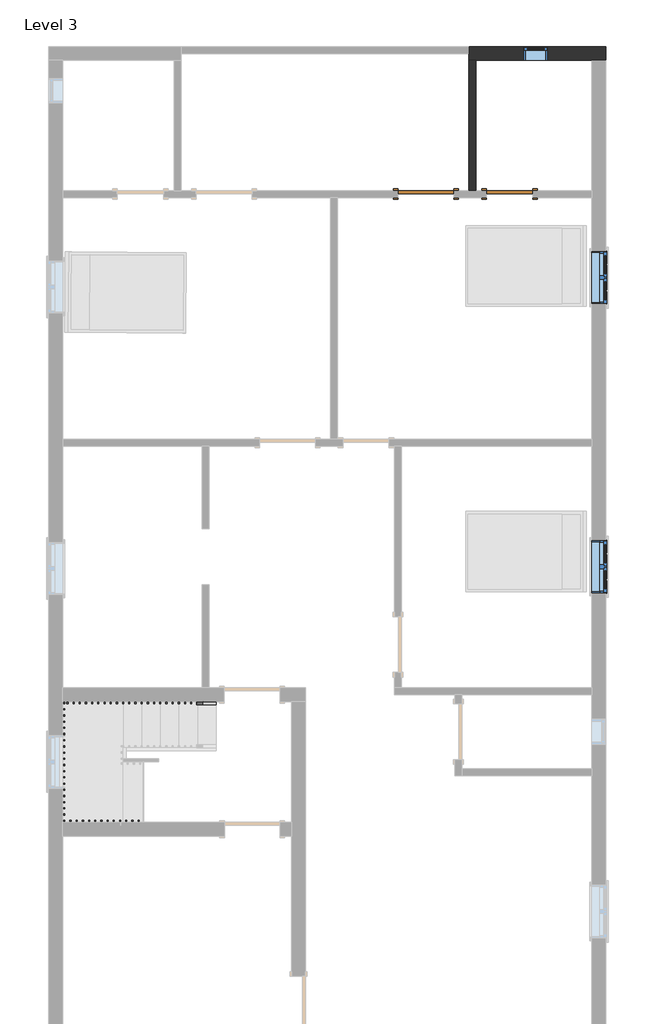
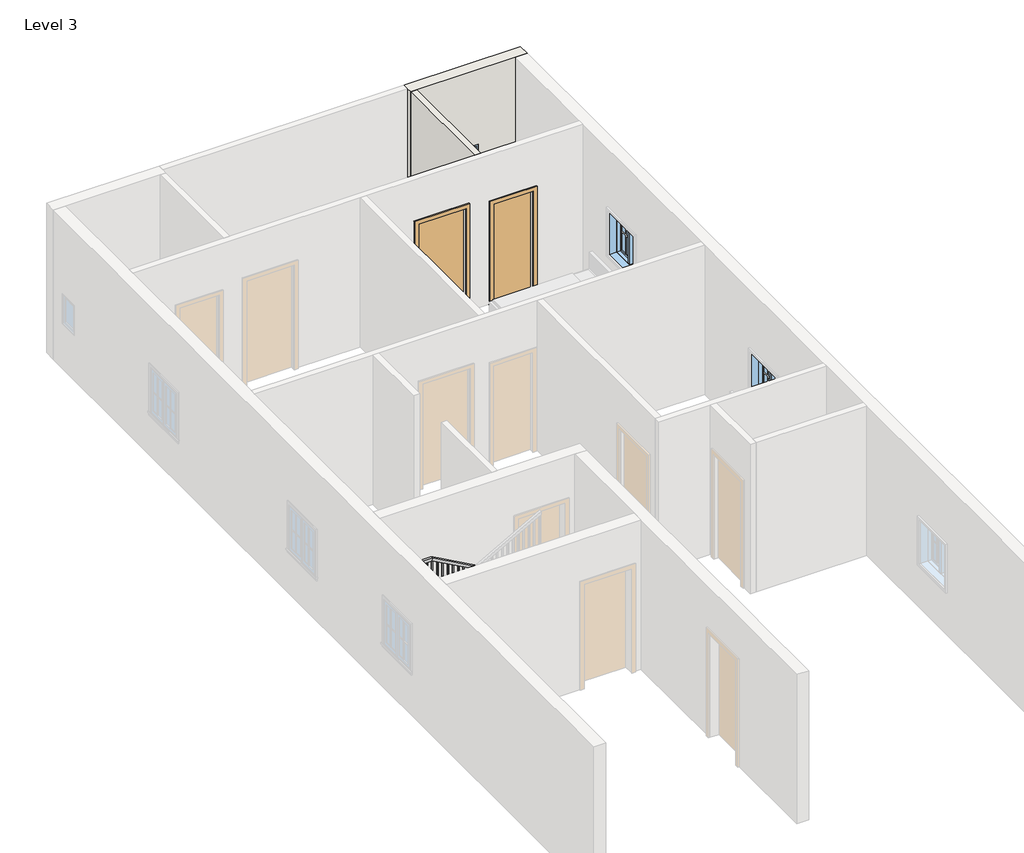
# One storey, part 2 of 3: 3 windows, 2 doors, 2 walls, 1 railing.
"""IFC4 building model written with IfcOpenShell, lengths in millimetres."""

from ifc_helpers import new_model, si_unit, frame, origin, place, context, project, spatial, polyline, outline, extrude, faceted_brep, transform, mapped, element, save
from components import door_f2b275c1, door_e5f9f3c4, window_aa618e30, window_339605e1

model = new_model("IFC4")

# Units and contexts
model_context = context("Model", 3, world=origin())
ifc_project = project(units=[si_unit("LENGTHUNIT", "METRE", prefix="MILLI")], contexts=[model_context])

# Site, building, storey
site = spatial("IfcSite", under=ifc_project)
building = spatial("IfcBuilding", under=site)
storey = spatial("IfcBuildingStorey", under=building, Name="Level 3", Elevation=3200.4)

# Doors
placement = place(None, origin())
door_shape = door_f2b275c1(model_context)
element("IfcDoor", 1, ObjectType="Single-Flush : 30\" x 80\"", at=placement, inside=storey, context=model_context, shape_type="MappedRepresentation", body=[
    mapped(door_shape, transform((1735.6084916, 8007.7072267, 3200.4), x_axis=(-1.0, 0.0, 0.0), y_axis=(0.0, -1.0, 0.0), z_axis=(0.0, 0.0, 1.0))),
])
door_2_shape = door_e5f9f3c4(model_context)
element("IfcDoor", 2, ObjectType="Single-Flush : 36\" x 84\"", at=placement, inside=storey, context=model_context, shape_type="MappedRepresentation", body=[
    mapped(door_2_shape, transform((364.0084916, 8007.7072267, 3200.4), x_axis=(1.0, 0.0, 0.0), y_axis=(0.0, 1.0, 0.0), z_axis=(0.0, 0.0, 1.0))),
])

# Railing
element("IfcRailing", 3, ObjectType="Handrail - Rectangular", at=placement, inside=storey, context=model_context, shape_type="SolidModel", body=[
    faceted_brep([(-3084.0415084, -367.9427733, 4284.1333333), (-3084.0415084, -367.9427733, 4226.020221), (-3084.0415084, -317.1427733, 4226.020221), (-3084.0415084, -317.1427733, 4284.1333333), (-4608.0415084, -367.9427733, 5130.8), (-4621.2051106, -367.9427733, 5080.0), (-4621.2051106, -317.1427733, 5080.0), (-4608.0415084, -317.1427733, 5130.8), (-5547.8415084, -367.9427733, 5130.8), (-5547.8415084, -367.9427733, 5080.0), (-5598.6415084, -317.1427733, 5080.0), (-5598.6415084, -317.1427733, 5130.8), (-5547.8415084, -2247.5427733, 5130.8), (-5547.8415084, -2247.5427733, 5080.0), (-5598.6415084, -2298.3427733, 5080.0), (-5598.6415084, -2298.3427733, 5130.8), (-4912.8415084, -2247.5427733, 5130.8), (-4899.6779062, -2247.5427733, 5080.0), (-4899.6779062, -2298.3427733, 5080.0), (-4912.8415084, -2298.3427733, 5130.8), (-3084.0415084, -2247.5427733, 6146.8), (-3084.0415084, -2298.3427733, 6146.8), (-3084.0415084, -2298.3427733, 6088.6868876), (-3084.0415084, -2247.5427733, 6088.6868876)], [[[0, 1, 2, 3]], [[1, 0, 4, 5]], [[2, 1, 5, 6]], [[3, 2, 6, 7]], [[0, 3, 7, 4]], [[5, 4, 8, 9]], [[6, 5, 9, 10]], [[7, 6, 10, 11]], [[4, 7, 11, 8]], [[9, 8, 12, 13]], [[10, 9, 13, 14]], [[11, 10, 14, 15]], [[8, 11, 15, 12]], [[13, 12, 16, 17]], [[14, 13, 17, 18]], [[15, 14, 18, 19]], [[12, 15, 19, 16]], [[20, 21, 22, 23]], [[17, 16, 20, 23]], [[18, 17, 23, 22]], [[19, 18, 22, 21]], [[16, 19, 21, 20]]]),
    extrude(outline(polyline([(6065.7563321, -3125.3165084), (6055.1729988, -3144.3665084), (5063.0666667, -3144.3665084), (5063.0666667, -3125.3165084), (6065.7563321, -3125.3165084)])), frame((0.0, -2282.4677733, 0.0), z_axis=(0.0, 1.0, 0.0), x_axis=(0.0, 0.0, 1.0)), (0.0, 0.0, 1.0), 19.05),
    extrude(outline(polyline([(6009.3118876, -3226.9165084), (5998.7285543, -3245.9665084), (5063.0666667, -3245.9665084), (5063.0666667, -3226.9165084), (6009.3118876, -3226.9165084)])), frame((0.0, -2282.4677733, 0.0), z_axis=(0.0, 1.0, 0.0), x_axis=(0.0, 0.0, 1.0)), (0.0, 0.0, 1.0), 19.05),
    extrude(outline(polyline([(5952.8674432, -3328.5165084), (5942.2841099, -3347.5665084), (5063.0666667, -3347.5665084), (5063.0666667, -3328.5165084), (5952.8674432, -3328.5165084)])), frame((0.0, -2282.4677733, 0.0), z_axis=(0.0, 1.0, 0.0), x_axis=(0.0, 0.0, 1.0)), (0.0, 0.0, 1.0), 19.05),
    extrude(outline(polyline([(5896.4229988, -3430.1165084), (5885.8396654, -3449.1665084), (4893.7333333, -3449.1665084), (4893.7333333, -3430.1165084), (5896.4229988, -3430.1165084)])), frame((0.0, -2282.4677733, 0.0), z_axis=(0.0, 1.0, 0.0), x_axis=(0.0, 0.0, 1.0)), (0.0, 0.0, 1.0), 19.05),
    extrude(outline(polyline([(5839.9785543, -3531.7165084), (5829.395221, -3550.7665084), (4893.7333333, -3550.7665084), (4893.7333333, -3531.7165084), (5839.9785543, -3531.7165084)])), frame((0.0, -2282.4677733, 0.0), z_axis=(0.0, 1.0, 0.0), x_axis=(0.0, 0.0, 1.0)), (0.0, 0.0, 1.0), 19.05),
    extrude(outline(polyline([(5783.5341099, -3633.3165084), (5772.9507765, -3652.3665084), (4893.7333333, -3652.3665084), (4893.7333333, -3633.3165084), (5783.5341099, -3633.3165084)])), frame((0.0, -2282.4677733, 0.0), z_axis=(0.0, 1.0, 0.0), x_axis=(0.0, 0.0, 1.0)), (0.0, 0.0, 1.0), 19.05),
    extrude(outline(polyline([(5727.0896654, -3734.9165084), (5716.5063321, -3753.9665084), (4724.4, -3753.9665084), (4724.4, -3734.9165084), (5727.0896654, -3734.9165084)])), frame((0.0, -2282.4677733, 0.0), z_axis=(0.0, 1.0, 0.0), x_axis=(0.0, 0.0, 1.0)), (0.0, 0.0, 1.0), 19.05),
    extrude(outline(polyline([(5670.645221, -3836.5165084), (5660.0618876, -3855.5665084), (4724.4, -3855.5665084), (4724.4, -3836.5165084), (5670.645221, -3836.5165084)])), frame((0.0, -2282.4677733, 0.0), z_axis=(0.0, 1.0, 0.0), x_axis=(0.0, 0.0, 1.0)), (0.0, 0.0, 1.0), 19.05),
    extrude(outline(polyline([(5614.2007765, -3938.1165084), (5603.6174432, -3957.1665084), (4724.4, -3957.1665084), (4724.4, -3938.1165084), (5614.2007765, -3938.1165084)])), frame((0.0, -2282.4677733, 0.0), z_axis=(0.0, 1.0, 0.0), x_axis=(0.0, 0.0, 1.0)), (0.0, 0.0, 1.0), 19.05),
    extrude(outline(polyline([(5557.7563321, -4039.7165084), (5547.1729988, -4058.7665084), (4555.0666667, -4058.7665084), (4555.0666667, -4039.7165084), (5557.7563321, -4039.7165084)])), frame((0.0, -2282.4677733, 0.0), z_axis=(0.0, 1.0, 0.0), x_axis=(0.0, 0.0, 1.0)), (0.0, 0.0, 1.0), 19.05),
    extrude(outline(polyline([(5501.3118876, -4141.3165084), (5490.7285543, -4160.3665084), (4555.0666667, -4160.3665084), (4555.0666667, -4141.3165084), (5501.3118876, -4141.3165084)])), frame((0.0, -2282.4677733, 0.0), z_axis=(0.0, 1.0, 0.0), x_axis=(0.0, 0.0, 1.0)), (0.0, 0.0, 1.0), 19.05),
    extrude(outline(polyline([(5444.8674432, -4242.9165084), (5434.2841099, -4261.9665084), (4555.0666667, -4261.9665084), (4555.0666667, -4242.9165084), (5444.8674432, -4242.9165084)])), frame((0.0, -2282.4677733, 0.0), z_axis=(0.0, 1.0, 0.0), x_axis=(0.0, 0.0, 1.0)), (0.0, 0.0, 1.0), 19.05),
    extrude(outline(polyline([(5388.4229988, -4344.5165084), (5377.8396654, -4363.5665084), (4385.7333333, -4363.5665084), (4385.7333333, -4344.5165084), (5388.4229988, -4344.5165084)])), frame((0.0, -2282.4677733, 0.0), z_axis=(0.0, 1.0, 0.0), x_axis=(0.0, 0.0, 1.0)), (0.0, 0.0, 1.0), 19.05),
    extrude(outline(polyline([(5331.9785543, -4446.1165084), (5321.395221, -4465.1665084), (4385.7333333, -4465.1665084), (4385.7333333, -4446.1165084), (5331.9785543, -4446.1165084)])), frame((0.0, -2282.4677733, 0.0), z_axis=(0.0, 1.0, 0.0), x_axis=(0.0, 0.0, 1.0)), (0.0, 0.0, 1.0), 19.05),
    extrude(outline(polyline([(5275.5341099, -4547.7165084), (5264.9507765, -4566.7665084), (4385.7333333, -4566.7665084), (4385.7333333, -4547.7165084), (5275.5341099, -4547.7165084)])), frame((0.0, -2282.4677733, 0.0), z_axis=(0.0, 1.0, 0.0), x_axis=(0.0, 0.0, 1.0)), (0.0, 0.0, 1.0), 19.05),
    extrude(outline(polyline([(5219.0896654, -4649.3165084), (5208.5063321, -4668.3665084), (4216.4, -4668.3665084), (4216.4, -4649.3165084), (5219.0896654, -4649.3165084)])), frame((0.0, -2282.4677733, 0.0), z_axis=(0.0, 1.0, 0.0), x_axis=(0.0, 0.0, 1.0)), (0.0, 0.0, 1.0), 19.05),
    extrude(outline(polyline([(5162.645221, -4750.9165084), (5152.0618876, -4769.9665084), (4216.4, -4769.9665084), (4216.4, -4750.9165084), (5162.645221, -4750.9165084)])), frame((0.0, -2282.4677733, 0.0), z_axis=(0.0, 1.0, 0.0), x_axis=(0.0, 0.0, 1.0)), (0.0, 0.0, 1.0), 19.05),
    extrude(outline(polyline([(5106.2007765, -4852.5165084), (5095.6174432, -4871.5665084), (4216.4, -4871.5665084), (4216.4, -4852.5165084), (5106.2007765, -4852.5165084)])), frame((0.0, -2282.4677733, 0.0), z_axis=(0.0, 1.0, 0.0), x_axis=(0.0, 0.0, 1.0)), (0.0, 0.0, 1.0), 19.05),
    extrude(outline(polyline([(-4973.1665084, -2282.4677733), (-4973.1665084, -2263.4177733), (-4954.1165084, -2263.4177733), (-4954.1165084, -2282.4677733), (-4973.1665084, -2282.4677733)])), frame((0.0, 0.0, 4216.4), z_axis=(0.0, 0.0, 1.0), x_axis=(1.0, 0.0, 0.0)), (0.0, 0.0, 1.0), 863.6),
    extrude(outline(polyline([(-5074.7665084, -2282.4677733), (-5074.7665084, -2263.4177733), (-5055.7165084, -2263.4177733), (-5055.7165084, -2282.4677733), (-5074.7665084, -2282.4677733)])), frame((0.0, 0.0, 4216.4), z_axis=(0.0, 0.0, 1.0), x_axis=(1.0, 0.0, 0.0)), (0.0, 0.0, 1.0), 863.6),
    extrude(outline(polyline([(-5176.3665084, -2282.4677733), (-5176.3665084, -2263.4177733), (-5157.3165084, -2263.4177733), (-5157.3165084, -2282.4677733), (-5176.3665084, -2282.4677733)])), frame((0.0, 0.0, 4216.4), z_axis=(0.0, 0.0, 1.0), x_axis=(1.0, 0.0, 0.0)), (0.0, 0.0, 1.0), 863.6),
    extrude(outline(polyline([(-5277.9665084, -2282.4677733), (-5277.9665084, -2263.4177733), (-5258.9165084, -2263.4177733), (-5258.9165084, -2282.4677733), (-5277.9665084, -2282.4677733)])), frame((0.0, 0.0, 4216.4), z_axis=(0.0, 0.0, 1.0), x_axis=(1.0, 0.0, 0.0)), (0.0, 0.0, 1.0), 863.6),
    extrude(outline(polyline([(-5379.5665084, -2282.4677733), (-5379.5665084, -2263.4177733), (-5360.5165084, -2263.4177733), (-5360.5165084, -2282.4677733), (-5379.5665084, -2282.4677733)])), frame((0.0, 0.0, 4216.4), z_axis=(0.0, 0.0, 1.0), x_axis=(1.0, 0.0, 0.0)), (0.0, 0.0, 1.0), 863.6),
    extrude(outline(polyline([(-5481.1665084, -2282.4677733), (-5481.1665084, -2263.4177733), (-5462.1165084, -2263.4177733), (-5462.1165084, -2282.4677733), (-5481.1665084, -2282.4677733)])), frame((0.0, 0.0, 4216.4), z_axis=(0.0, 0.0, 1.0), x_axis=(1.0, 0.0, 0.0)), (0.0, 0.0, 1.0), 863.6),
    extrude(outline(polyline([(-5582.7665084, -2161.8177733), (-5563.7165084, -2161.8177733), (-5563.7165084, -2180.8677733), (-5582.7665084, -2180.8677733), (-5582.7665084, -2161.8177733)])), frame((0.0, 0.0, 4216.4), z_axis=(0.0, 0.0, 1.0), x_axis=(1.0, 0.0, 0.0)), (0.0, 0.0, 1.0), 863.6),
    extrude(outline(polyline([(-5582.7665084, -2060.2177733), (-5563.7165084, -2060.2177733), (-5563.7165084, -2079.2677733), (-5582.7665084, -2079.2677733), (-5582.7665084, -2060.2177733)])), frame((0.0, 0.0, 4216.4), z_axis=(0.0, 0.0, 1.0), x_axis=(1.0, 0.0, 0.0)), (0.0, 0.0, 1.0), 863.6),
    extrude(outline(polyline([(-5582.7665084, -1958.6177733), (-5563.7165084, -1958.6177733), (-5563.7165084, -1977.6677733), (-5582.7665084, -1977.6677733), (-5582.7665084, -1958.6177733)])), frame((0.0, 0.0, 4216.4), z_axis=(0.0, 0.0, 1.0), x_axis=(1.0, 0.0, 0.0)), (0.0, 0.0, 1.0), 863.6),
    extrude(outline(polyline([(-5582.7665084, -1857.0177733), (-5563.7165084, -1857.0177733), (-5563.7165084, -1876.0677733), (-5582.7665084, -1876.0677733), (-5582.7665084, -1857.0177733)])), frame((0.0, 0.0, 4216.4), z_axis=(0.0, 0.0, 1.0), x_axis=(1.0, 0.0, 0.0)), (0.0, 0.0, 1.0), 863.6),
    extrude(outline(polyline([(-5582.7665084, -1755.4177733), (-5563.7165084, -1755.4177733), (-5563.7165084, -1774.4677733), (-5582.7665084, -1774.4677733), (-5582.7665084, -1755.4177733)])), frame((0.0, 0.0, 4216.4), z_axis=(0.0, 0.0, 1.0), x_axis=(1.0, 0.0, 0.0)), (0.0, 0.0, 1.0), 863.6),
    extrude(outline(polyline([(-5582.7665084, -1653.8177733), (-5563.7165084, -1653.8177733), (-5563.7165084, -1672.8677733), (-5582.7665084, -1672.8677733), (-5582.7665084, -1653.8177733)])), frame((0.0, 0.0, 4216.4), z_axis=(0.0, 0.0, 1.0), x_axis=(1.0, 0.0, 0.0)), (0.0, 0.0, 1.0), 863.6),
    extrude(outline(polyline([(-5582.7665084, -1552.2177733), (-5563.7165084, -1552.2177733), (-5563.7165084, -1571.2677733), (-5582.7665084, -1571.2677733), (-5582.7665084, -1552.2177733)])), frame((0.0, 0.0, 4216.4), z_axis=(0.0, 0.0, 1.0), x_axis=(1.0, 0.0, 0.0)), (0.0, 0.0, 1.0), 863.6),
    extrude(outline(polyline([(-5582.7665084, -1450.6177733), (-5563.7165084, -1450.6177733), (-5563.7165084, -1469.6677733), (-5582.7665084, -1469.6677733), (-5582.7665084, -1450.6177733)])), frame((0.0, 0.0, 4216.4), z_axis=(0.0, 0.0, 1.0), x_axis=(1.0, 0.0, 0.0)), (0.0, 0.0, 1.0), 863.6),
    extrude(outline(polyline([(-5582.7665084, -1349.0177733), (-5563.7165084, -1349.0177733), (-5563.7165084, -1368.0677733), (-5582.7665084, -1368.0677733), (-5582.7665084, -1349.0177733)])), frame((0.0, 0.0, 4216.4), z_axis=(0.0, 0.0, 1.0), x_axis=(1.0, 0.0, 0.0)), (0.0, 0.0, 1.0), 863.6),
    extrude(outline(polyline([(-5582.7665084, -1247.4177733), (-5563.7165084, -1247.4177733), (-5563.7165084, -1266.4677733), (-5582.7665084, -1266.4677733), (-5582.7665084, -1247.4177733)])), frame((0.0, 0.0, 4216.4), z_axis=(0.0, 0.0, 1.0), x_axis=(1.0, 0.0, 0.0)), (0.0, 0.0, 1.0), 863.6),
    extrude(outline(polyline([(-5582.7665084, -1145.8177733), (-5563.7165084, -1145.8177733), (-5563.7165084, -1164.8677733), (-5582.7665084, -1164.8677733), (-5582.7665084, -1145.8177733)])), frame((0.0, 0.0, 4216.4), z_axis=(0.0, 0.0, 1.0), x_axis=(1.0, 0.0, 0.0)), (0.0, 0.0, 1.0), 863.6),
    extrude(outline(polyline([(-5582.7665084, -1044.2177733), (-5563.7165084, -1044.2177733), (-5563.7165084, -1063.2677733), (-5582.7665084, -1063.2677733), (-5582.7665084, -1044.2177733)])), frame((0.0, 0.0, 4216.4), z_axis=(0.0, 0.0, 1.0), x_axis=(1.0, 0.0, 0.0)), (0.0, 0.0, 1.0), 863.6),
    extrude(outline(polyline([(-5582.7665084, -942.6177733), (-5563.7165084, -942.6177733), (-5563.7165084, -961.6677733), (-5582.7665084, -961.6677733), (-5582.7665084, -942.6177733)])), frame((0.0, 0.0, 4216.4), z_axis=(0.0, 0.0, 1.0), x_axis=(1.0, 0.0, 0.0)), (0.0, 0.0, 1.0), 863.6),
    extrude(outline(polyline([(-5582.7665084, -841.0177733), (-5563.7165084, -841.0177733), (-5563.7165084, -860.0677733), (-5582.7665084, -860.0677733), (-5582.7665084, -841.0177733)])), frame((0.0, 0.0, 4216.4), z_axis=(0.0, 0.0, 1.0), x_axis=(1.0, 0.0, 0.0)), (0.0, 0.0, 1.0), 863.6),
    extrude(outline(polyline([(-5582.7665084, -739.4177733), (-5563.7165084, -739.4177733), (-5563.7165084, -758.4677733), (-5582.7665084, -758.4677733), (-5582.7665084, -739.4177733)])), frame((0.0, 0.0, 4216.4), z_axis=(0.0, 0.0, 1.0), x_axis=(1.0, 0.0, 0.0)), (0.0, 0.0, 1.0), 863.6),
    extrude(outline(polyline([(-5582.7665084, -637.8177733), (-5563.7165084, -637.8177733), (-5563.7165084, -656.8677733), (-5582.7665084, -656.8677733), (-5582.7665084, -637.8177733)])), frame((0.0, 0.0, 4216.4), z_axis=(0.0, 0.0, 1.0), x_axis=(1.0, 0.0, 0.0)), (0.0, 0.0, 1.0), 863.6),
    extrude(outline(polyline([(-5582.7665084, -536.2177733), (-5563.7165084, -536.2177733), (-5563.7165084, -555.2677733), (-5582.7665084, -555.2677733), (-5582.7665084, -536.2177733)])), frame((0.0, 0.0, 4216.4), z_axis=(0.0, 0.0, 1.0), x_axis=(1.0, 0.0, 0.0)), (0.0, 0.0, 1.0), 863.6),
    extrude(outline(polyline([(-5582.7665084, -434.6177733), (-5563.7165084, -434.6177733), (-5563.7165084, -453.6677733), (-5582.7665084, -453.6677733), (-5582.7665084, -434.6177733)])), frame((0.0, 0.0, 4216.4), z_axis=(0.0, 0.0, 1.0), x_axis=(1.0, 0.0, 0.0)), (0.0, 0.0, 1.0), 863.6),
    extrude(outline(polyline([(-5512.9165084, -333.0177733), (-5512.9165084, -352.0677733), (-5531.9665084, -352.0677733), (-5531.9665084, -333.0177733), (-5512.9165084, -333.0177733)])), frame((0.0, 0.0, 4216.4), z_axis=(0.0, 0.0, 1.0), x_axis=(1.0, 0.0, 0.0)), (0.0, 0.0, 1.0), 863.6),
    extrude(outline(polyline([(-5411.3165084, -333.0177733), (-5411.3165084, -352.0677733), (-5430.3665084, -352.0677733), (-5430.3665084, -333.0177733), (-5411.3165084, -333.0177733)])), frame((0.0, 0.0, 4216.4), z_axis=(0.0, 0.0, 1.0), x_axis=(1.0, 0.0, 0.0)), (0.0, 0.0, 1.0), 863.6),
    extrude(outline(polyline([(-5309.7165084, -333.0177733), (-5309.7165084, -352.0677733), (-5328.7665084, -352.0677733), (-5328.7665084, -333.0177733), (-5309.7165084, -333.0177733)])), frame((0.0, 0.0, 4216.4), z_axis=(0.0, 0.0, 1.0), x_axis=(1.0, 0.0, 0.0)), (0.0, 0.0, 1.0), 863.6),
    extrude(outline(polyline([(-5208.1165084, -333.0177733), (-5208.1165084, -352.0677733), (-5227.1665084, -352.0677733), (-5227.1665084, -333.0177733), (-5208.1165084, -333.0177733)])), frame((0.0, 0.0, 4216.4), z_axis=(0.0, 0.0, 1.0), x_axis=(1.0, 0.0, 0.0)), (0.0, 0.0, 1.0), 863.6),
    extrude(outline(polyline([(-5106.5165084, -333.0177733), (-5106.5165084, -352.0677733), (-5125.5665084, -352.0677733), (-5125.5665084, -333.0177733), (-5106.5165084, -333.0177733)])), frame((0.0, 0.0, 4216.4), z_axis=(0.0, 0.0, 1.0), x_axis=(1.0, 0.0, 0.0)), (0.0, 0.0, 1.0), 863.6),
    extrude(outline(polyline([(-5004.9165084, -333.0177733), (-5004.9165084, -352.0677733), (-5023.9665084, -352.0677733), (-5023.9665084, -333.0177733), (-5004.9165084, -333.0177733)])), frame((0.0, 0.0, 4216.4), z_axis=(0.0, 0.0, 1.0), x_axis=(1.0, 0.0, 0.0)), (0.0, 0.0, 1.0), 863.6),
    extrude(outline(polyline([(-4903.3165084, -333.0177733), (-4903.3165084, -352.0677733), (-4922.3665084, -352.0677733), (-4922.3665084, -333.0177733), (-4903.3165084, -333.0177733)])), frame((0.0, 0.0, 4216.4), z_axis=(0.0, 0.0, 1.0), x_axis=(1.0, 0.0, 0.0)), (0.0, 0.0, 1.0), 863.6),
    extrude(outline(polyline([(-4801.7165084, -333.0177733), (-4801.7165084, -352.0677733), (-4820.7665084, -352.0677733), (-4820.7665084, -333.0177733), (-4801.7165084, -333.0177733)])), frame((0.0, 0.0, 4216.4), z_axis=(0.0, 0.0, 1.0), x_axis=(1.0, 0.0, 0.0)), (0.0, 0.0, 1.0), 863.6),
    extrude(outline(polyline([(-4700.1165084, -333.0177733), (-4700.1165084, -352.0677733), (-4719.1665084, -352.0677733), (-4719.1665084, -333.0177733), (-4700.1165084, -333.0177733)])), frame((0.0, 0.0, 4216.4), z_axis=(0.0, 0.0, 1.0), x_axis=(1.0, 0.0, 0.0)), (0.0, 0.0, 1.0), 863.6),
    extrude(outline(polyline([(5067.395221, -4598.5165084), (5077.9785543, -4617.5665084), (4216.4, -4617.5665084), (4216.4, -4598.5165084), (5067.395221, -4598.5165084)])), frame((0.0, -352.0677733, 0.0), z_axis=(0.0, 1.0, 0.0), x_axis=(0.0, 0.0, 1.0)), (0.0, 0.0, 1.0), 19.05),
    extrude(outline(polyline([(5010.9507765, -4496.9165084), (5021.5341099, -4515.9665084), (4047.0666667, -4515.9665084), (4047.0666667, -4496.9165084), (5010.9507765, -4496.9165084)])), frame((0.0, -352.0677733, 0.0), z_axis=(0.0, 1.0, 0.0), x_axis=(0.0, 0.0, 1.0)), (0.0, 0.0, 1.0), 19.05),
    extrude(outline(polyline([(4954.5063321, -4395.3165084), (4965.0896654, -4414.3665084), (4047.0666667, -4414.3665084), (4047.0666667, -4395.3165084), (4954.5063321, -4395.3165084)])), frame((0.0, -352.0677733, 0.0), z_axis=(0.0, 1.0, 0.0), x_axis=(0.0, 0.0, 1.0)), (0.0, 0.0, 1.0), 19.05),
    extrude(outline(polyline([(4898.0618876, -4293.7165084), (4908.645221, -4312.7665084), (4047.0666667, -4312.7665084), (4047.0666667, -4293.7165084), (4898.0618876, -4293.7165084)])), frame((0.0, -352.0677733, 0.0), z_axis=(0.0, 1.0, 0.0), x_axis=(0.0, 0.0, 1.0)), (0.0, 0.0, 1.0), 19.05),
    extrude(outline(polyline([(4841.6174432, -4192.1165084), (4852.2007765, -4211.1665084), (3877.7333333, -4211.1665084), (3877.7333333, -4192.1165084), (4841.6174432, -4192.1165084)])), frame((0.0, -352.0677733, 0.0), z_axis=(0.0, 1.0, 0.0), x_axis=(0.0, 0.0, 1.0)), (0.0, 0.0, 1.0), 19.05),
    extrude(outline(polyline([(4785.1729988, -4090.5165084), (4795.7563321, -4109.5665084), (3877.7333333, -4109.5665084), (3877.7333333, -4090.5165084), (4785.1729988, -4090.5165084)])), frame((0.0, -352.0677733, 0.0), z_axis=(0.0, 1.0, 0.0), x_axis=(0.0, 0.0, 1.0)), (0.0, 0.0, 1.0), 19.05),
    extrude(outline(polyline([(4728.7285543, -3988.9165084), (4739.3118876, -4007.9665084), (3877.7333333, -4007.9665084), (3877.7333333, -3988.9165084), (4728.7285543, -3988.9165084)])), frame((0.0, -352.0677733, 0.0), z_axis=(0.0, 1.0, 0.0), x_axis=(0.0, 0.0, 1.0)), (0.0, 0.0, 1.0), 19.05),
    extrude(outline(polyline([(4672.2841099, -3887.3165084), (4682.8674432, -3906.3665084), (3708.4, -3906.3665084), (3708.4, -3887.3165084), (4672.2841099, -3887.3165084)])), frame((0.0, -352.0677733, 0.0), z_axis=(0.0, 1.0, 0.0), x_axis=(0.0, 0.0, 1.0)), (0.0, 0.0, 1.0), 19.05),
    extrude(outline(polyline([(4615.8396654, -3785.7165084), (4626.4229988, -3804.7665084), (3708.4, -3804.7665084), (3708.4, -3785.7165084), (4615.8396654, -3785.7165084)])), frame((0.0, -352.0677733, 0.0), z_axis=(0.0, 1.0, 0.0), x_axis=(0.0, 0.0, 1.0)), (0.0, 0.0, 1.0), 19.05),
    extrude(outline(polyline([(4559.395221, -3684.1165084), (4569.9785543, -3703.1665084), (3708.4, -3703.1665084), (3708.4, -3684.1165084), (4559.395221, -3684.1165084)])), frame((0.0, -352.0677733, 0.0), z_axis=(0.0, 1.0, 0.0), x_axis=(0.0, 0.0, 1.0)), (0.0, 0.0, 1.0), 19.05),
    extrude(outline(polyline([(4502.9507765, -3582.5165084), (4513.5341099, -3601.5665084), (3539.0666667, -3601.5665084), (3539.0666667, -3582.5165084), (4502.9507765, -3582.5165084)])), frame((0.0, -352.0677733, 0.0), z_axis=(0.0, 1.0, 0.0), x_axis=(0.0, 0.0, 1.0)), (0.0, 0.0, 1.0), 19.05),
    extrude(outline(polyline([(4446.5063321, -3480.9165084), (4457.0896654, -3499.9665084), (3539.0666667, -3499.9665084), (3539.0666667, -3480.9165084), (4446.5063321, -3480.9165084)])), frame((0.0, -352.0677733, 0.0), z_axis=(0.0, 1.0, 0.0), x_axis=(0.0, 0.0, 1.0)), (0.0, 0.0, 1.0), 19.05),
    extrude(outline(polyline([(4390.0618876, -3379.3165084), (4400.645221, -3398.3665084), (3539.0666667, -3398.3665084), (3539.0666667, -3379.3165084), (4390.0618876, -3379.3165084)])), frame((0.0, -352.0677733, 0.0), z_axis=(0.0, 1.0, 0.0), x_axis=(0.0, 0.0, 1.0)), (0.0, 0.0, 1.0), 19.05),
    extrude(outline(polyline([(4333.6174432, -3277.7165084), (4344.2007765, -3296.7665084), (3369.7333333, -3296.7665084), (3369.7333333, -3277.7165084), (4333.6174432, -3277.7165084)])), frame((0.0, -352.0677733, 0.0), z_axis=(0.0, 1.0, 0.0), x_axis=(0.0, 0.0, 1.0)), (0.0, 0.0, 1.0), 19.05),
    extrude(outline(polyline([(4277.1729988, -3176.1165084), (4287.7563321, -3195.1665084), (3369.7333333, -3195.1665084), (3369.7333333, -3176.1165084), (4277.1729988, -3176.1165084)])), frame((0.0, -352.0677733, 0.0), z_axis=(0.0, 1.0, 0.0), x_axis=(0.0, 0.0, 1.0)), (0.0, 0.0, 1.0), 19.05),
    extrude(outline(polyline([(-5582.7665084, -2263.4177733), (-5563.7165084, -2263.4177733), (-5563.7165084, -2282.4677733), (-5582.7665084, -2282.4677733), (-5582.7665084, -2263.4177733)])), frame((0.0, 0.0, 4216.4), z_axis=(0.0, 0.0, 1.0), x_axis=(1.0, 0.0, 0.0)), (0.0, 0.0, 1.0), 863.6),
    extrude(outline(polyline([(-5563.7165084, -333.0177733), (-5563.7165084, -352.0677733), (-5582.7665084, -352.0677733), (-5582.7665084, -333.0177733), (-5563.7165084, -333.0177733)])), frame((0.0, 0.0, 4216.4), z_axis=(0.0, 0.0, 1.0), x_axis=(1.0, 0.0, 0.0)), (0.0, 0.0, 1.0), 863.6),
    extrude(outline(polyline([(6088.6868876, -3084.0415084), (6078.1035543, -3103.0915084), (5063.0666667, -3103.0915084), (5063.0666667, -3084.0415084), (6088.6868876, -3084.0415084)])), frame((0.0, -2282.4677733, 0.0), z_axis=(0.0, 1.0, 0.0), x_axis=(0.0, 0.0, 1.0)), (0.0, 0.0, 1.0), 19.05),
    extrude(outline(polyline([(4226.020221, -3084.0415084), (4236.6035543, -3103.0915084), (3369.7333333, -3103.0915084), (3369.7333333, -3084.0415084), (4226.020221, -3084.0415084)])), frame((0.0, -352.0677733, 0.0), z_axis=(0.0, 1.0, 0.0), x_axis=(0.0, 0.0, 1.0)), (0.0, 0.0, 1.0), 19.05),
])

# Walls
element("IfcWall", 4, ObjectType="WALL4.5\"", at=placement, inside=storey, context=model_context, shape_type="SweptSolid", body=[
    extrude(outline(polyline([(1068.8584916, 8064.8572267), (1068.8584916, 10198.4572267), (1183.1584916, 10198.4572267), (1183.1584916, 8064.8572267), (1068.8584916, 8064.8572267)])), frame((0.0, 0.0, 3200.4), z_axis=(0.0, 0.0, 1.0), x_axis=(1.0, 0.0, 0.0)), (0.0, 0.0, 1.0), 3048.0),
])
element("IfcWall", 5, ObjectType="WALL9\"", at=placement, inside=storey, context=model_context, shape_type="Brep", body=[
    faceted_brep([(1068.8584916, 10198.4572267, 3200.4), (1183.1584916, 10198.4572267, 3200.4), (3088.1584916, 10198.4572267, 3200.4), (3316.7584916, 10198.4572267, 3200.4), (3316.7584916, 10198.4572267, 6248.4), (3088.1584916, 10198.4572267, 6248.4), (1183.1584916, 10198.4572267, 6248.4), (1068.8584916, 10198.4572267, 6248.4), (2367.4334916, 10198.4572267, 4724.4), (2367.4334916, 10198.4572267, 4114.8), (1961.0334916, 10198.4572267, 4114.8), (1961.0334916, 10198.4572267, 4724.4), (1068.8584916, 10427.0572267, 3200.4), (1068.8584916, 10427.0572267, 6248.4), (3316.7584916, 10427.0572267, 6248.4), (3316.7584916, 10427.0572267, 3200.4), (2367.4334916, 10427.0572267, 4724.4), (1961.0334916, 10427.0572267, 4724.4), (1961.0334916, 10427.0572267, 4114.8), (2367.4334916, 10427.0572267, 4114.8), (1068.8584916, 10312.7572267, 3200.4), (1068.8584916, 10312.7572267, 6248.4)], [[[0, 1, 2, 3, 4, 5, 6, 7], [8, 9, 10, 11]], [[12, 13, 14, 15], [16, 17, 18, 19]], [[3, 2, 1, 0, 20, 12, 15]], [[4, 3, 15, 14]], [[0, 7, 21, 13, 12, 20]], [[9, 8, 16, 19]], [[10, 9, 19, 18]], [[11, 10, 18, 17]], [[8, 11, 17, 16]], [[7, 6, 5, 4, 14, 13, 21]]]),
])

# Windows
window_shape = window_aa618e30(model_context)
element("IfcWindow", 6, ObjectType="Fixed : 16\" x 24\"", at=placement, inside=storey, context=model_context, shape_type="MappedRepresentation", body=[
    mapped(window_shape, transform((2202.3334916, 10312.7572267, 3200.4), x_axis=(1.0, 0.0, 0.0), y_axis=(0.0, 1.0, 0.0), z_axis=(0.0, 0.0, 1.0))),
])
window_2_shape = window_339605e1(model_context)
element("IfcWindow", 7, ObjectType="Window-Casement-Double : 34\" x 36\"", at=placement, inside=storey, context=model_context, shape_type="MappedRepresentation", body=[
    mapped(window_2_shape, transform((3202.4584916, 6636.1072267, 3200.4), x_axis=(0.0, -1.0, 0.0), y_axis=(1.0, 0.0, 0.0), z_axis=(0.0, 0.0, 1.0))),
])
element("IfcWindow", 8, ObjectType="Window-Casement-Double : 34\" x 36\"", at=placement, inside=storey, context=model_context, shape_type="MappedRepresentation", body=[
    mapped(window_2_shape, transform((3202.4584916, 1892.6572267, 3200.4), x_axis=(0.0, -1.0, 0.0), y_axis=(1.0, 0.0, 0.0), z_axis=(0.0, 0.0, 1.0))),
])

save(model, "model.ifc")

# Revit data of these elements
# Type "Single-Flush : 30\" x 80\""
#   Type Mark = "5"
#   Construction Type Id = "MDOOR"
#   Assembly Code = "C1020"
#   Analytic Construction = "Metal"
#   Thickness = 0' - 2"
#   Heat Transfer Coefficient (U) = 0.651978 BTU/(h·ft²·°F)
#   Height = 6' - 8"
#   Trim Projection Ext = 0' - 1"
#   Trim Projection Int = 0' - 1"
#   Trim Width = 0' - 3"
#   Width = 2' - 6"
#   Define Thermal Properties by = 1
#   Define Thermal Properties by = 1
#   Door Material = Door - Panel
#   Frame Material = Door - Frame
#   Visual Light Transmittance = 0
#   Solar Heat Gain Coefficient = 0
#   Function = (empty or 0)
#   Wall Closure = (empty or 0)
# Type "Single-Flush : 36\" x 84\""
#   Type Mark = "1"
#   Construction Type Id = "MDOOR"
#   Assembly Code = "C1020"
#   Analytic Construction = "Metal"
#   Thickness = 0' - 2"
#   Heat Transfer Coefficient (U) = 0.651978 BTU/(h·ft²·°F)
#   Height = 7' - 0"
#   Trim Projection Ext = 0' - 1"
#   Trim Projection Int = 0' - 1"
#   Trim Width = 0' - 3"
#   Width = 3' - 0"
#   Define Thermal Properties by = 1
#   Define Thermal Properties by = 1
#   Door Material = Door - Panel
#   Frame Material = Door - Frame
#   Visual Light Transmittance = 0
#   Solar Heat Gain Coefficient = 0
#   Function = (empty or 0)
#   Wall Closure = (empty or 0)
# Type "Handrail - Rectangular"
#   Assembly Code = "C2010400"
#   built-in parameter 1008612 = 0.0416667 (stored number, unit not read)
#   built-in parameter 1008611 = 0.0416667 (stored number, unit not read)
#   built-in parameter 1008609 = 0.333333 (stored number, unit not read)
#   built-in parameter 1008604 = 0.166667 (stored number, unit not read)
#   built-in parameter 1008603 = 0.166667 (stored number, unit not read)
#   Railing Height = 3' - 0"
#   built-in parameter 1008630 = 2
#   built-in parameter 1008610 = 2
#   built-in parameter 1008618 = Baluster - Square : 3/4"
# Type "WALL4.5\""
#   Assembly Code = "B2010"
#   Layers, outside or top first: 0' - 4 1/2" no material (function 1)
# Type "WALL9\""
#   Assembly Code = "B2010"
#   Layers, outside or top first: 0' - 9" no material (function 1)
# Type "Fixed : 16\" x 24\""
#   Type Mark = "4"
#   Construction Type Id = "GSP4R"
#   Assembly Code = "B2020100"
#   Analytic Construction = "1/8 in Pilkington single glazing"
#   Visual Light Transmittance = 0.9
#   Solar Heat Gain Coefficient = 0.78
#   Heat Transfer Coefficient (U) = 0.6496 BTU/(h·ft²·°F)
#   Height = 2' - 0"
#   Default Sill Height = 3' - 0"
#   Width = 1' - 4"
#   Window Inset = 0' - 0 3/4"
#   Define Thermal Properties by = 1
#   Define Thermal Properties by = 1
#   Glass Pane Material = Glass
#   Sash Material = Sash
#   Wall Closure = (empty or 0)
# Type "Window-Casement-Double : 34\" x 36\""
#   Type Mark = "14"
#   Fire Rating = "0.5h"
#   Assembly Code = "B2020100"
#   Analytic Construction = "Double glazing - domestic"
#   Frame Extension [instance default] = 0' - 0 1/4"
#   Window Inset [instance default] = 0' - 0"
#   Wall Thickness [instance default] = 0' - 6"
#   Interior Wall Closure [instance default] = 0' - 2 1/4"
#   Half Width = 1' - 5"
#   Visual Light Transmittance = 0.81
#   Thermal Resistance (R) = 1.8146 (h·ft²·°F)/BTU
#   Solar Heat Gain Coefficient = 0.76
#   Rough Width = 2' - 10 1/2"
#   Rough Height = 3' - 0 1/2"
#   Height = 3' - 0"
#   Heat Transfer Coefficient (U) = 0.5511 BTU/(h·ft²·°F)
#   Exterior Wall Closure [instance default] = 0' - 1 1/4"
#   Extension Jamb [instance default] = 0' - 2 1/4"
#   Default Sill Height = 3' - 0"
#   Width = 2' - 10"
#   Define Thermal Properties by = 0
#   Muntin Visibility = yes
#   Interior Trim Visibility [instance default] = yes
#   Exterior Trim Visibility [instance default] = yes
#   Extension Jamb Visibility [instance default] = yes
#   Interior Trim Material = Wood - Stained
#   Muntin Pattern = Muntin Pattern_2x2 : Muntin Pattern_2x2
#   Interior Trim = Trim-Window-Interior-Flat : Picture Frame
#   Interior Frame Material = Wood - Stained
#   Glass Panel Material = Glass
#   Exterior Trim Material = Clad - White
#   Exterior Trim = Trim-Window-Exterior-Flat : with Sill
#   Exterior Frame Material = Clad - White
#   Wall Closure = (empty or 0)
# Element 1 (IfcDoor, "Single-Flush : 30\" x 80\"")
#   Phase Created = New Construction
#   Materials on its faces: "Door - Frame", "Door - Panel"
# Element 2 (IfcDoor, "Single-Flush : 36\" x 84\"")
#   Phase Created = New Construction
#   Materials on its faces: "Door - Frame", "Door - Panel"
# Element 3 (IfcRailing, "Handrail - Rectangular")
#   Phase Created = New Construction
# Element 4 (IfcWall, "WALL4.5\"")
#   Top Offset = 0' - 0"
#   Base Offset = 0' - 0"
#   Unconnected Height = 10' - 0"
#   wall height = 10' - 0"
#   Phase Created = New Construction
#   Base Constraint = Level 3
#   Materials on its faces: "Default Wall", "Wood Planks"
# Element 5 (IfcWall, "WALL9\"")
#   Top Offset = 0' - 0"
#   Base Offset = 0' - 0"
#   Unconnected Height = 10' - 0"
#   wall height = 10' - 0"
#   Phase Created = New Construction
#   Base Constraint = Level 3
#   Materials on its faces: "Default Wall", "Wood Planks"
# Element 6 (IfcWindow, "Fixed : 16\" x 24\"")
#   Mark = "11"
#   Phase Created = New Construction
#   Materials on its faces: "Sash", "Glass"
# Element 7 (IfcWindow, "Window-Casement-Double : 34\" x 36\"")
#   Mark = "13"
#   Window Inset = 0' - 0"
#   Interior Wall Closure = 0' - 2 1/4"
#   Frame Extension = 0' - 0 1/4"
#   Exterior Wall Closure = 0' - 1 1/4"
#   Interior Trim Visibility = yes
#   Exterior Trim Visibility = yes
#   Phase Created = New Construction
#   Materials on its faces: "Wood - Stained", "Glass", "Clad - White"
# Element 8 (IfcWindow, "Window-Casement-Double : 34\" x 36\"")
#   Mark = "14"
#   Window Inset = 0' - 0"
#   Interior Wall Closure = 0' - 2 1/4"
#   Frame Extension = 0' - 0 1/4"
#   Exterior Wall Closure = 0' - 1 1/4"
#   Interior Trim Visibility = yes
#   Exterior Trim Visibility = yes
#   Phase Created = New Construction
#   Materials on its faces: "Wood - Stained", "Glass", "Clad - White"
# Materials
#   "Door - Panel": class "Wood", colour RGB 210 159 95, transparency 0, Cost = 0
#   "Door - Frame": colour RGB 118 70 51, transparency 0, Cost = 0
#   "Glass": class "Glass", colour RGB 0 128 192, transparency 0.75, Description = "Soda Lime Glass", Cost = 0
#   "Sash": class "Wood", colour RGB 224 178 126, transparency 0, Cost = 0
#   "Wood - Stained": class "Wood", colour RGB 224 178 126, transparency 0, Cost = 0
#   "Clad - White": class "Wood", colour RGB 242 242 238, transparency 0, Cost = 0
#   "Default Wall": colour RGB 128 128 128, transparency 0, Cost = 0
#   "Wood Planks": class "Wood", colour RGB 193 160 115, transparency 0, Description = "Physical material.", Cost = 0
